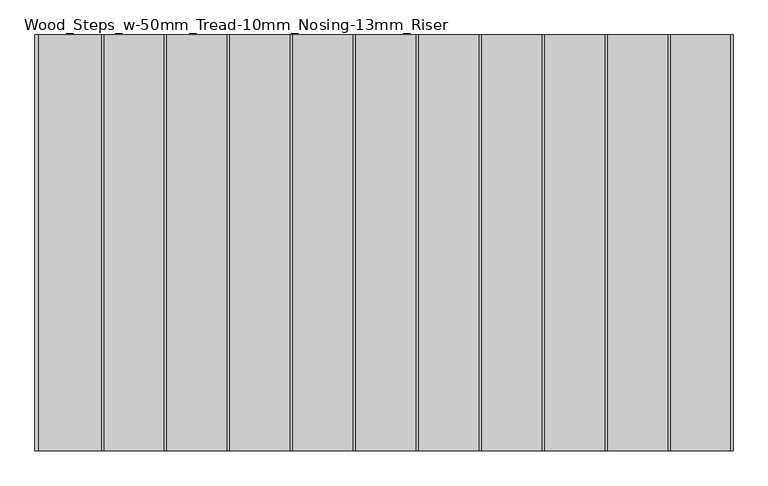
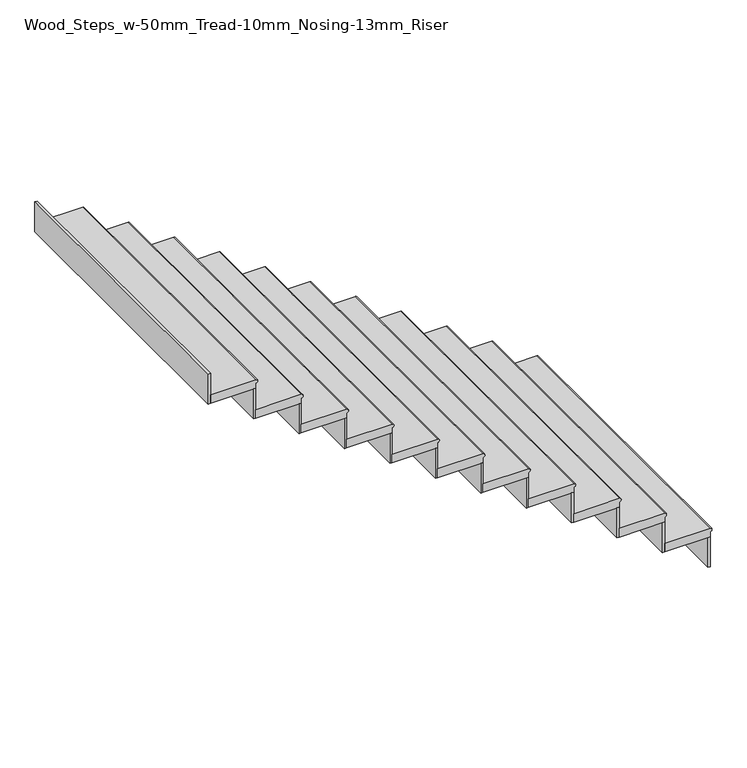
"""IFC4 building model written with IfcOpenShell, lengths in millimetres: stair flight geometry, Wood_Steps_w-50mm_Tread-10mm_Nosing-13mm_Riser."""

from ifc_helpers import new_model, si_unit, point, frame, frame_2d, origin, place, context, project, spatial, polyline, circle_curve, trimmed, segment, composite_curve, outline, extrude, source, transform, mapped, element, save


def wood_steps_w_50mm_tread_10mm_nosing_13mm_riser_e3607291(model_context):
    return source(origin(), model_context, "Body", "SweptSolid", [
        extrude(outline(composite_curve([segment(polyline([(2260.8695652, 2217.0011137), (2260.8695652, 1967.0011137), (2210.8695652, 1967.0011137), (2210.8695652, 2217.0011137), (2240.8695652, 2217.0011137)]), True, "CONTINUOUS"), segment(trimmed(circle_curve(frame_2d((2250.8695652, 2217.0011137)), 10.0), [point((2240.8695652, 2217.0011137))], [point((2260.8695652, 2217.0011137))], False, "CARTESIAN"), True, "CONTINUOUS")], self_intersect=False)), frame((0.0, -8065.821978, 0.0), z_axis=(0.0, 1.0, 0.0), x_axis=(0.0, 0.0, 1.0)), (0.0, 0.0, 1.0), 1651.0),
        extrude(outline(polyline([(2204.5011137, -6414.821978), (2217.0011137, -6414.821978), (2217.0011137, -8065.821978), (2204.5011137, -8065.821978), (2204.5011137, -6414.821978)])), frame((0.0, 0.0, 2036.9565217), z_axis=(0.0, 0.0, 1.0), x_axis=(1.0, 0.0, 0.0)), (0.0, 0.0, 1.0), 173.9130435),
        extrude(outline(polyline([(1954.5011137, -6414.821978), (1967.0011137, -6414.821978), (1967.0011137, -8065.821978), (1954.5011137, -8065.821978), (1954.5011137, -6414.821978)])), frame((0.0, 0.0, 2210.8695652), z_axis=(0.0, 0.0, 1.0), x_axis=(1.0, 0.0, 0.0)), (0.0, 0.0, 1.0), 173.9130435),
        extrude(outline(composite_curve([segment(polyline([(2434.7826087, 1967.0011137), (2434.7826087, 1717.0011137), (2384.7826087, 1717.0011137), (2384.7826087, 1967.0011137), (2414.7826087, 1967.0011137)]), True, "CONTINUOUS"), segment(trimmed(circle_curve(frame_2d((2424.7826087, 1967.0011137)), 10.0), [point((2414.7826087, 1967.0011137))], [point((2434.7826087, 1967.0011137))], False, "CARTESIAN"), True, "CONTINUOUS")], self_intersect=False)), frame((0.0, -8065.821978, 0.0), z_axis=(0.0, 1.0, 0.0), x_axis=(0.0, 0.0, 1.0)), (0.0, 0.0, 1.0), 1651.0),
        extrude(outline(polyline([(1704.5011137, -6414.821978), (1717.0011137, -6414.821978), (1717.0011137, -8065.821978), (1704.5011137, -8065.821978), (1704.5011137, -6414.821978)])), frame((0.0, 0.0, 2384.7826087), z_axis=(0.0, 0.0, 1.0), x_axis=(1.0, 0.0, 0.0)), (0.0, 0.0, 1.0), 173.9130435),
        extrude(outline(composite_curve([segment(polyline([(2608.6956522, 1717.0011137), (2608.6956522, 1467.0011137), (2558.6956522, 1467.0011137), (2558.6956522, 1717.0011137), (2588.6956522, 1717.0011137)]), True, "CONTINUOUS"), segment(trimmed(circle_curve(frame_2d((2598.6956522, 1717.0011137)), 10.0), [point((2588.6956522, 1717.0011137))], [point((2608.6956522, 1717.0011137))], False, "CARTESIAN"), True, "CONTINUOUS")], self_intersect=False)), frame((0.0, -8065.821978, 0.0), z_axis=(0.0, 1.0, 0.0), x_axis=(0.0, 0.0, 1.0)), (0.0, 0.0, 1.0), 1651.0),
        extrude(outline(polyline([(1454.5011137, -6414.821978), (1467.0011137, -6414.821978), (1467.0011137, -8065.821978), (1454.5011137, -8065.821978), (1454.5011137, -6414.821978)])), frame((0.0, 0.0, 2558.6956522), z_axis=(0.0, 0.0, 1.0), x_axis=(1.0, 0.0, 0.0)), (0.0, 0.0, 1.0), 173.9130435),
        extrude(outline(composite_curve([segment(polyline([(2782.6086957, 1467.0011137), (2782.6086957, 1217.0011137), (2732.6086957, 1217.0011137), (2732.6086957, 1467.0011137), (2762.6086957, 1467.0011137)]), True, "CONTINUOUS"), segment(trimmed(circle_curve(frame_2d((2772.6086957, 1467.0011137)), 10.0), [point((2762.6086957, 1467.0011137))], [point((2782.6086957, 1467.0011137))], False, "CARTESIAN"), True, "CONTINUOUS")], self_intersect=False)), frame((0.0, -8065.821978, 0.0), z_axis=(0.0, 1.0, 0.0), x_axis=(0.0, 0.0, 1.0)), (0.0, 0.0, 1.0), 1651.0),
        extrude(outline(polyline([(1204.5011137, -6414.821978), (1217.0011137, -6414.821978), (1217.0011137, -8065.821978), (1204.5011137, -8065.821978), (1204.5011137, -6414.821978)])), frame((0.0, 0.0, 2732.6086957), z_axis=(0.0, 0.0, 1.0), x_axis=(1.0, 0.0, 0.0)), (0.0, 0.0, 1.0), 173.9130435),
        extrude(outline(composite_curve([segment(polyline([(2956.5217391, 1217.0011137), (2956.5217391, 967.0011137), (2906.5217391, 967.0011137), (2906.5217391, 1217.0011137), (2936.5217391, 1217.0011137)]), True, "CONTINUOUS"), segment(trimmed(circle_curve(frame_2d((2946.5217391, 1217.0011137)), 10.0), [point((2936.5217391, 1217.0011137))], [point((2956.5217391, 1217.0011137))], False, "CARTESIAN"), True, "CONTINUOUS")], self_intersect=False)), frame((0.0, -8065.821978, 0.0), z_axis=(0.0, 1.0, 0.0), x_axis=(0.0, 0.0, 1.0)), (0.0, 0.0, 1.0), 1651.0),
        extrude(outline(polyline([(954.5011137, -6414.821978), (967.0011137, -6414.821978), (967.0011137, -8065.821978), (954.5011137, -8065.821978), (954.5011137, -6414.821978)])), frame((0.0, 0.0, 2906.5217391), z_axis=(0.0, 0.0, 1.0), x_axis=(1.0, 0.0, 0.0)), (0.0, 0.0, 1.0), 173.9130435),
        extrude(outline(composite_curve([segment(polyline([(3130.4347826, 967.0011137), (3130.4347826, 717.0011137), (3080.4347826, 717.0011137), (3080.4347826, 967.0011137), (3110.4347826, 967.0011137)]), True, "CONTINUOUS"), segment(trimmed(circle_curve(frame_2d((3120.4347826, 967.0011137)), 10.0), [point((3110.4347826, 967.0011137))], [point((3130.4347826, 967.0011137))], False, "CARTESIAN"), True, "CONTINUOUS")], self_intersect=False)), frame((0.0, -8065.821978, 0.0), z_axis=(0.0, 1.0, 0.0), x_axis=(0.0, 0.0, 1.0)), (0.0, 0.0, 1.0), 1651.0),
        extrude(outline(polyline([(704.5011137, -6414.821978), (717.0011137, -6414.821978), (717.0011137, -8065.821978), (704.5011137, -8065.821978), (704.5011137, -6414.821978)])), frame((0.0, 0.0, 3080.4347826), z_axis=(0.0, 0.0, 1.0), x_axis=(1.0, 0.0, 0.0)), (0.0, 0.0, 1.0), 173.9130435),
        extrude(outline(composite_curve([segment(polyline([(3304.3478261, 717.0011137), (3304.3478261, 467.0011137), (3254.3478261, 467.0011137), (3254.3478261, 717.0011137), (3284.3478261, 717.0011137)]), True, "CONTINUOUS"), segment(trimmed(circle_curve(frame_2d((3294.3478261, 717.0011137)), 10.0), [point((3284.3478261, 717.0011137))], [point((3304.3478261, 717.0011137))], False, "CARTESIAN"), True, "CONTINUOUS")], self_intersect=False)), frame((0.0, -8065.821978, 0.0), z_axis=(0.0, 1.0, 0.0), x_axis=(0.0, 0.0, 1.0)), (0.0, 0.0, 1.0), 1651.0),
        extrude(outline(polyline([(454.5011137, -6414.821978), (467.0011137, -6414.821978), (467.0011137, -8065.821978), (454.5011137, -8065.821978), (454.5011137, -6414.821978)])), frame((0.0, 0.0, 3254.3478261), z_axis=(0.0, 0.0, 1.0), x_axis=(1.0, 0.0, 0.0)), (0.0, 0.0, 1.0), 173.9130435),
        extrude(outline(composite_curve([segment(polyline([(3478.2608696, 467.0011137), (3478.2608696, 217.0011137), (3428.2608696, 217.0011137), (3428.2608696, 467.0011137), (3458.2608696, 467.0011137)]), True, "CONTINUOUS"), segment(trimmed(circle_curve(frame_2d((3468.2608696, 467.0011137)), 10.0), [point((3458.2608696, 467.0011137))], [point((3478.2608696, 467.0011137))], False, "CARTESIAN"), True, "CONTINUOUS")], self_intersect=False)), frame((0.0, -8065.821978, 0.0), z_axis=(0.0, 1.0, 0.0), x_axis=(0.0, 0.0, 1.0)), (0.0, 0.0, 1.0), 1651.0),
        extrude(outline(polyline([(204.5011137, -6414.821978), (217.0011137, -6414.821978), (217.0011137, -8065.821978), (204.5011137, -8065.821978), (204.5011137, -6414.821978)])), frame((0.0, 0.0, 3428.2608696), z_axis=(0.0, 0.0, 1.0), x_axis=(1.0, 0.0, 0.0)), (0.0, 0.0, 1.0), 173.9130435),
        extrude(outline(composite_curve([segment(polyline([(3652.173913, 217.0011137), (3652.173913, -32.9988863), (3602.173913, -32.9988863), (3602.173913, 217.0011137), (3632.173913, 217.0011137)]), True, "CONTINUOUS"), segment(trimmed(circle_curve(frame_2d((3642.173913, 217.0011137)), 10.0), [point((3632.173913, 217.0011137))], [point((3652.173913, 217.0011137))], False, "CARTESIAN"), True, "CONTINUOUS")], self_intersect=False)), frame((0.0, -8065.821978, 0.0), z_axis=(0.0, 1.0, 0.0), x_axis=(0.0, 0.0, 1.0)), (0.0, 0.0, 1.0), 1651.0),
        extrude(outline(polyline([(-45.4988863, -6414.821978), (-32.9988863, -6414.821978), (-32.9988863, -8065.821978), (-45.4988863, -8065.821978), (-45.4988863, -6414.821978)])), frame((0.0, 0.0, 3602.173913), z_axis=(0.0, 0.0, 1.0), x_axis=(1.0, 0.0, 0.0)), (0.0, 0.0, 1.0), 173.9130435),
        extrude(outline(composite_curve([segment(polyline([(3826.0869565, -32.9988863), (3826.0869565, -282.9988863), (3776.0869565, -282.9988863), (3776.0869565, -32.9988863), (3806.0869565, -32.9988863)]), True, "CONTINUOUS"), segment(trimmed(circle_curve(frame_2d((3816.0869565, -32.9988863)), 10.0), [point((3806.0869565, -32.9988863))], [point((3826.0869565, -32.9988863))], False, "CARTESIAN"), True, "CONTINUOUS")], self_intersect=False)), frame((0.0, -8065.821978, 0.0), z_axis=(0.0, 1.0, 0.0), x_axis=(0.0, 0.0, 1.0)), (0.0, 0.0, 1.0), 1651.0),
        extrude(outline(polyline([(-295.4988863, -6414.821978), (-282.9988863, -6414.821978), (-282.9988863, -8065.821978), (-295.4988863, -8065.821978), (-295.4988863, -6414.821978)])), frame((0.0, 0.0, 3776.0869565), z_axis=(0.0, 0.0, 1.0), x_axis=(1.0, 0.0, 0.0)), (0.0, 0.0, 1.0), 173.9130435),
        extrude(outline(polyline([(-545.4988863, -6414.821978), (-532.9988863, -6414.821978), (-532.9988863, -8065.821978), (-545.4988863, -8065.821978), (-545.4988863, -6414.821978)])), frame((0.0, 0.0, 3950.0), z_axis=(0.0, 0.0, 1.0), x_axis=(1.0, 0.0, 0.0)), (0.0, 0.0, 1.0), 173.9130435),
        extrude(outline(composite_curve([segment(polyline([(4000.0, -282.9988863), (4000.0, -532.9988863), (3950.0, -532.9988863), (3950.0, -282.9988863), (3980.0, -282.9988863)]), True, "CONTINUOUS"), segment(trimmed(circle_curve(frame_2d((3990.0, -282.9988863)), 10.0), [point((3980.0, -282.9988863))], [point((4000.0, -282.9988863))], False, "CARTESIAN"), True, "CONTINUOUS")], self_intersect=False)), frame((0.0, -8065.821978, 0.0), z_axis=(0.0, 1.0, 0.0), x_axis=(0.0, 0.0, 1.0)), (0.0, 0.0, 1.0), 1651.0),
    ])


if __name__ == "__main__":
    model = new_model("IFC4")
    model_context = context("Model", 3, world=origin())
    ifc_project = project(units=[si_unit("LENGTHUNIT", "METRE", prefix="MILLI")], contexts=[model_context])
    site = spatial("IfcSite", under=ifc_project)
    building = spatial("IfcBuilding", under=site)
    placement = place(None, origin())
    wood_steps_w_50mm_tread_10mm_nosing_13mm_riser_shape = wood_steps_w_50mm_tread_10mm_nosing_13mm_riser_e3607291(model_context)
    element("IfcStairFlight", 1, ObjectType="Wood_Steps_w-50mm_Tread-10mm_Nosing-13mm_Riser", at=placement, inside=building, context=model_context, shape_type="MappedRepresentation", body=[
        mapped(wood_steps_w_50mm_tread_10mm_nosing_13mm_riser_shape, transform((0.0, 0.0, 0.0), x_axis=(1.0, 0.0, 0.0), y_axis=(0.0, 1.0, 0.0), z_axis=(0.0, 0.0, 1.0))),
    ])
    save(model, "model.ifc")

# Revit data of these elements
# Element 1 (IfcStairFlight, "Wood_Steps_w-50mm_Tread-10mm_Nosing-13mm_Riser")
#   Materials on its faces: "Oak Flooring"
# Materials
#   "Oak Flooring": class "Wood", colour RGB 212 179 113, transparency 0, Description = "Quercus Rubra", Cost = 0
